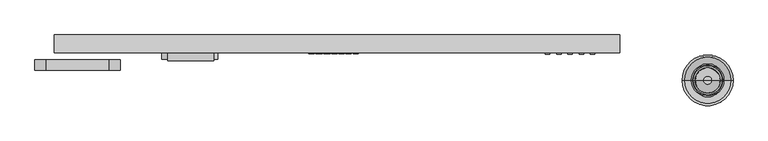
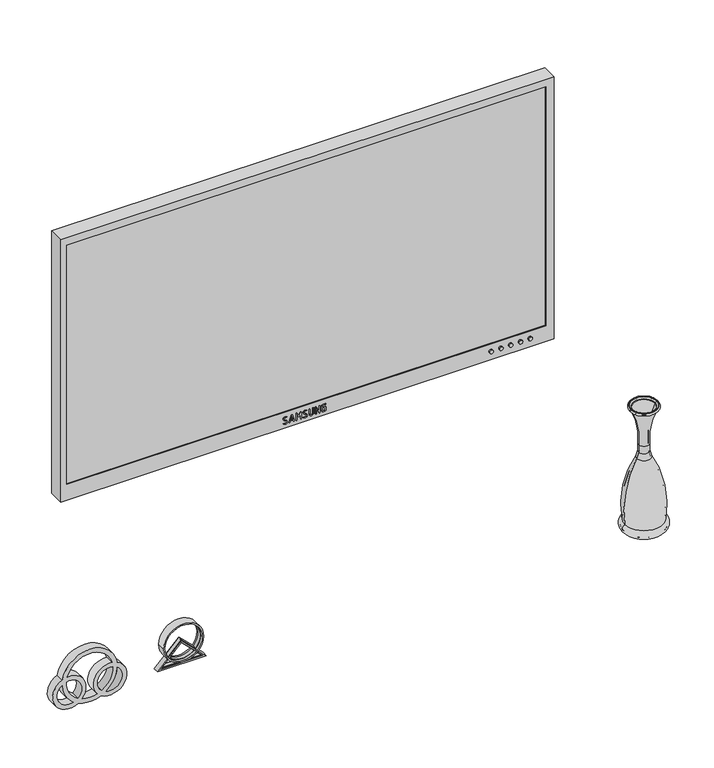
"""IFC4 building model written with IfcOpenShell, lengths in millimetres: furniture geometry."""

from ifc_helpers import new_model, si_unit, point, frame, frame_2d, origin, place, context, project, spatial, polyline, circle_curve, ellipse_curve, trimmed, segment, composite_curve, outline, extrude, faceted_brep, source, transform, mapped, element, save
from ifc_brep_helpers import plane_surface, cylinder_surface, revolved_surface, advanced_brep


def furniture_f593881e(model_context):
    return source(origin(), model_context, "Body", "SolidModel", [
        advanced_brep(
        [(1619.2140368, -127.8036565, 1022.4850219), (1533.669479, -127.8036565, 1022.4850219), (1532.6909812, -127.8036565, 1028.7350001), (1620.1925345, -127.8036565, 1028.7350001), (1617.5743227, -127.8036565, 1022.2360813), (1535.309193, -127.8036565, 1022.2360813), (1616.2567383, -127.8036565, 1021.2783955), (1536.6267775, -127.8036565, 1021.2783955), (1593.5125539, -127.8036565, 899.7037334), (1559.3709618, -127.8036565, 899.7037334), (1593.5125539, -127.8036565, 874.0721871), (1559.3709618, -127.8036565, 874.0721871), (1598.9034231, -127.8036565, 853.9701278), (1553.9800927, -127.8036565, 853.9701278), (1638.1633362, -127.8036565, 641.294886), (1514.7201795, -127.8036565, 641.294886), (1640.3690284, -127.8036565, 613.767552), (1512.5144873, -127.8036565, 613.767552), (1576.4417579, -127.8036565, 613.767552), (1634.3411967, -127.8036565, 617.0820621), (1518.5423191, -127.8036565, 617.0820621), (1576.4417579, -127.8036565, 617.0820621), (1632.4749509, -127.8036565, 637.0427782), (1520.4085649, -127.8036565, 637.0427782), (1594.3579463, -127.8036565, 851.8571485), (1558.5255695, -127.8036565, 851.8571485), (1588.5125539, -127.8036565, 873.6724497), (1564.3709618, -127.8036565, 873.6724497), (1588.5125539, -127.8036565, 899.4734315), (1564.3709618, -127.8036565, 899.4734315), (1611.5170749, -127.8036565, 1023.1126524), (1541.3664409, -127.8036565, 1023.1126524), (1612.9045122, -127.8036565, 1024.5000897), (1539.9790036, -127.8036565, 1024.5000897), (1616.8480298, -127.8036565, 1028.5337475), (1536.035486, -127.8036565, 1028.5337475)],
        [
            (0, 1, circle_curve(frame((1576.4417579, -127.8036565, 1022.4850219), z_axis=(0.0, 0.0, 1.0), x_axis=(-1.0, 0.0, 0.0)), 42.7722789)),
            (1, 2, circle_curve(frame((1533.4520615, -127.8036565, 1025.652569), z_axis=(0.0, 1.0, 0.0), x_axis=(1.0, 0.0, 0.0)), 3.175)),
            (2, 3, circle_curve(frame((1576.4417579, -127.8036565, 1028.7350001), z_axis=(0.0, 0.0, -1.0), x_axis=(-1.0, 0.0, 0.0)), 43.7507767)),
            (3, 0, circle_curve(frame((1619.4314542, -127.8036565, 1025.652569), z_axis=(0.0, 1.0, 0.0), x_axis=(-1.0, 0.0, 0.0)), 3.175)),
            (1, 0, circle_curve(frame((1576.4417579, -127.8036565, 1022.4850219), z_axis=(0.0, 0.0, 1.0), x_axis=(-1.0, 0.0, 0.0)), 42.7722789)),
            (3, 2, circle_curve(frame((1576.4417579, -127.8036565, 1028.7350001), z_axis=(0.0, 0.0, -1.0), x_axis=(-1.0, 0.0, 0.0)), 43.7507767)),
            (4, 5, circle_curve(frame((1576.4417579, -127.8036565, 1022.2360813), z_axis=(0.0, 0.0, 1.0), x_axis=(-1.0, 0.0, 0.0)), 41.1325648)),
            (5, 1, circle_curve(frame((1576.9707974, -127.8036565, 1302.1760704), z_axis=(0.0, 1.0, 0.0), x_axis=(1.0, 0.0, 0.0)), 283.0231206)),
            (0, 4, circle_curve(frame((1575.9127183, -127.8036565, 1302.1760704), z_axis=(0.0, 1.0, 0.0), x_axis=(-1.0, 0.0, 0.0)), 283.0231206)),
            (5, 4, circle_curve(frame((1576.4417579, -127.8036565, 1022.2360813), z_axis=(0.0, 0.0, 1.0), x_axis=(-1.0, 0.0, 0.0)), 41.1325648)),
            (6, 7, circle_curve(frame((1576.4417579, -127.8036565, 1021.2783955), z_axis=(0.0, 0.0, 1.0), x_axis=(-1.0, 0.0, 0.0)), 39.8149804)),
            (7, 5, circle_curve(frame((1535.0499641, -127.8036565, 1020.4942245), z_axis=(0.0, -1.0, 0.0), x_axis=(-1.0, 0.0, 0.0)), 1.7610408)),
            (4, 6, circle_curve(frame((1617.8335517, -127.8036565, 1020.4942245), z_axis=(0.0, -1.0, 0.0), x_axis=(1.0, 0.0, 0.0)), 1.7610408)),
            (7, 6, circle_curve(frame((1576.4417579, -127.8036565, 1021.2783955), z_axis=(0.0, 0.0, 1.0), x_axis=(-1.0, 0.0, 0.0)), 39.8149804)),
            (8, 9, circle_curve(frame((1576.4417579, -127.8036565, 899.7037334), z_axis=(0.0, 0.0, 1.0), x_axis=(-1.0, 0.0, 0.0)), 17.0707961)),
            (9, 7, circle_curve(frame((1334.1949035, -127.8036565, 920.6062281), z_axis=(0.0, -1.0, 0.0), x_axis=(1.0, 0.0, 0.0)), 226.1441389)),
            (6, 8, circle_curve(frame((1818.6886123, -127.8036565, 920.6062281), z_axis=(0.0, -1.0, 0.0), x_axis=(-1.0, 0.0, 0.0)), 226.1441389)),
            (9, 8, circle_curve(frame((1576.4417579, -127.8036565, 899.7037334), z_axis=(0.0, 0.0, 1.0), x_axis=(-1.0, 0.0, 0.0)), 17.0707961)),
            (10, 11, circle_curve(frame((1576.4417579, -127.8036565, 874.0721871), z_axis=(0.0, 0.0, 1.0), x_axis=(-1.0, 0.0, 0.0)), 17.0707961)),
            (11, 9),
            (8, 10),
            (11, 10, circle_curve(frame((1576.4417579, -127.8036565, 874.0721871), z_axis=(0.0, 0.0, 1.0), x_axis=(-1.0, 0.0, 0.0)), 17.0707961)),
            (12, 13, circle_curve(frame((1576.4417579, -127.8036565, 853.9701278), z_axis=(0.0, 0.0, 1.0), x_axis=(-1.0, 0.0, 0.0)), 22.4616652)),
            (13, 11, circle_curve(frame((1457.0512652, -127.8036565, 890.737891), z_axis=(0.0, -1.0, 0.0), x_axis=(1.0, 0.0, 0.0)), 103.6680569)),
            (10, 12, circle_curve(frame((1695.8322506, -127.8036565, 890.737891), z_axis=(0.0, -1.0, 0.0), x_axis=(-1.0, 0.0, 0.0)), 103.6680569)),
            (13, 12, circle_curve(frame((1576.4417579, -127.8036565, 853.9701278), z_axis=(0.0, 0.0, 1.0), x_axis=(-1.0, 0.0, 0.0)), 22.4616652)),
            (14, 15, circle_curve(frame((1576.4417579, -127.8036565, 641.294886), z_axis=(0.0, 0.0, 1.0), x_axis=(-1.0, 0.0, 0.0)), 61.7215784)),
            (15, 13, circle_curve(frame((1852.0874628, -127.8036565, 688.9781015), z_axis=(0.0, 1.0, 0.0), x_axis=(1.0, 0.0, 0.0)), 340.7203735)),
            (12, 14, circle_curve(frame((1300.7960529, -127.8036565, 688.9781015), z_axis=(0.0, 1.0, 0.0), x_axis=(-1.0, 0.0, 0.0)), 340.7203735)),
            (15, 14, circle_curve(frame((1576.4417579, -127.8036565, 641.294886), z_axis=(0.0, 0.0, 1.0), x_axis=(-1.0, 0.0, 0.0)), 61.7215784)),
            (16, 17, circle_curve(frame((1576.4417579, -127.8036565, 613.767552), z_axis=(0.0, 0.0, 1.0), x_axis=(-1.0, 0.0, 0.0)), 63.9272705)),
            (17, 15, circle_curve(frame((1519.5200125, -127.8036565, 627.058253), z_axis=(0.0, 1.0, 0.0), x_axis=(1.0, 0.0, 0.0)), 15.0239847)),
            (14, 16, circle_curve(frame((1633.3635033, -127.8036565, 627.058253), z_axis=(0.0, 1.0, 0.0), x_axis=(-1.0, 0.0, 0.0)), 15.0239847)),
            (17, 16, circle_curve(frame((1576.4417579, -127.8036565, 613.767552), z_axis=(0.0, 0.0, 1.0), x_axis=(-1.0, 0.0, 0.0)), 63.9272705)),
            (18, 17),
            (16, 18),
            (19, 20, circle_curve(frame((1576.4417579, -127.8036565, 617.0820621), z_axis=(0.0, 0.0, 1.0), x_axis=(-1.0, 0.0, 0.0)), 57.8994388)),
            (20, 21),
            (21, 19),
            (20, 19, circle_curve(frame((1576.4417579, -127.8036565, 617.0820621), z_axis=(0.0, 0.0, 1.0), x_axis=(-1.0, 0.0, 0.0)), 57.8994388)),
            (22, 23, circle_curve(frame((1576.4417579, -127.8036565, 637.0427782), z_axis=(0.0, 0.0, 1.0), x_axis=(-1.0, 0.0, 0.0)), 56.033193)),
            (23, 20, circle_curve(frame((1519.5200125, -127.8036565, 627.058253), z_axis=(0.0, -1.0, 0.0), x_axis=(1.0, 0.0, 0.0)), 10.0239847)),
            (19, 22, circle_curve(frame((1633.3635033, -127.8036565, 627.058253), z_axis=(0.0, -1.0, 0.0), x_axis=(-1.0, 0.0, 0.0)), 10.0239847)),
            (23, 22, circle_curve(frame((1576.4417579, -127.8036565, 637.0427782), z_axis=(0.0, 0.0, 1.0), x_axis=(-1.0, 0.0, 0.0)), 56.033193)),
            (24, 25, circle_curve(frame((1576.4417579, -127.8036565, 851.8571485), z_axis=(0.0, 0.0, 1.0), x_axis=(-1.0, 0.0, 0.0)), 17.9161884)),
            (25, 23, circle_curve(frame((1852.0874628, -127.8036565, 688.9781015), z_axis=(0.0, -1.0, 0.0), x_axis=(1.0, 0.0, 0.0)), 335.7203735)),
            (22, 24, circle_curve(frame((1300.7960529, -127.8036565, 688.9781015), z_axis=(0.0, -1.0, 0.0), x_axis=(-1.0, 0.0, 0.0)), 335.7203735)),
            (25, 24, circle_curve(frame((1576.4417579, -127.8036565, 851.8571485), z_axis=(0.0, 0.0, 1.0), x_axis=(-1.0, 0.0, 0.0)), 17.9161884)),
            (26, 27, circle_curve(frame((1576.4417579, -127.8036565, 873.6724497), z_axis=(0.0, 0.0, 1.0), x_axis=(-1.0, 0.0, 0.0)), 12.0707961)),
            (27, 25, circle_curve(frame((1457.0512652, -127.8036565, 890.737891), z_axis=(0.0, 1.0, 0.0), x_axis=(1.0, 0.0, 0.0)), 108.6680569)),
            (24, 26, circle_curve(frame((1695.8322506, -127.8036565, 890.737891), z_axis=(0.0, 1.0, 0.0), x_axis=(-1.0, 0.0, 0.0)), 108.6680569)),
            (27, 26, circle_curve(frame((1576.4417579, -127.8036565, 873.6724497), z_axis=(0.0, 0.0, 1.0), x_axis=(-1.0, 0.0, 0.0)), 12.0707961)),
            (28, 29, circle_curve(frame((1576.4417579, -127.8036565, 899.4734315), z_axis=(0.0, 0.0, 1.0), x_axis=(-1.0, 0.0, 0.0)), 12.0707961)),
            (29, 27),
            (26, 28),
            (29, 28, circle_curve(frame((1576.4417579, -127.8036565, 899.4734315), z_axis=(0.0, 0.0, 1.0), x_axis=(-1.0, 0.0, 0.0)), 12.0707961)),
            (30, 31, circle_curve(frame((1576.4417579, -127.8036565, 1023.1126524), z_axis=(0.0, 0.0, 1.0), x_axis=(-1.0, 0.0, 0.0)), 35.075317)),
            (31, 29, circle_curve(frame((1334.1949035, -127.8036565, 920.6062281), z_axis=(0.0, 1.0, 0.0), x_axis=(1.0, 0.0, 0.0)), 231.1441389)),
            (28, 30, circle_curve(frame((1818.6886123, -127.8036565, 920.6062281), z_axis=(0.0, 1.0, 0.0), x_axis=(-1.0, 0.0, 0.0)), 231.1441389)),
            (31, 30, circle_curve(frame((1576.4417579, -127.8036565, 1023.1126524), z_axis=(0.0, 0.0, 1.0), x_axis=(-1.0, 0.0, 0.0)), 35.075317)),
            (32, 33, circle_curve(frame((1576.4417579, -127.8036565, 1024.5000897), z_axis=(0.0, 0.0, 1.0), x_axis=(-1.0, 0.0, 0.0)), 36.4627543)),
            (33, 31),
            (30, 32),
            (33, 32, circle_curve(frame((1576.4417579, -127.8036565, 1024.5000897), z_axis=(0.0, 0.0, 1.0), x_axis=(-1.0, 0.0, 0.0)), 36.4627543)),
            (34, 35, circle_curve(frame((1576.4417579, -127.8036565, 1028.5337475), z_axis=(0.0, 0.0, 1.0), x_axis=(-1.0, 0.0, 0.0)), 40.4062719)),
            (35, 33, circle_curve(frame((1535.7876985, -127.8036565, 1024.3469724), z_axis=(0.0, 1.0, 0.0), x_axis=(-1.0, 0.0, 0.0)), 4.1941011)),
            (32, 34, circle_curve(frame((1617.0958173, -127.8036565, 1024.3469724), z_axis=(0.0, 1.0, 0.0), x_axis=(1.0, 0.0, 0.0)), 4.1941011)),
            (35, 34, circle_curve(frame((1576.4417579, -127.8036565, 1028.5337475), z_axis=(0.0, 0.0, 1.0), x_axis=(-1.0, 0.0, 0.0)), 40.4062719)),
            (2, 35, circle_curve(frame((1636.2916403, -127.8036565, 2722.5250067), z_axis=(0.0, -1.0, 0.0), x_axis=(1.0, 0.0, 0.0)), 1696.9554157)),
            (34, 3, circle_curve(frame((1516.5918754, -127.8036565, 2722.5250067), z_axis=(0.0, -1.0, 0.0), x_axis=(-1.0, 0.0, 0.0)), 1696.9554157)),
        ],
        [
            revolved_surface(trimmed(ellipse_curve(frame((1533.4520615, -127.8036565, 1025.652569), z_axis=(0.0, -1.0, 0.0), x_axis=(1.0, 0.0, 0.0)), 3.175, 3.175), [point((1532.6909812, -127.8036565, 1028.7350001))], [point((1533.669479, -127.8036565, 1022.4850219))], True, "CARTESIAN"), (1576.4417579, -127.8036565, 620.0444967), (0.0, 0.0, -1.0)),
            revolved_surface(trimmed(ellipse_curve(frame((1576.9707974, -127.8036565, 1302.1760704), z_axis=(0.0, -1.0, 0.0), x_axis=(1.0, 0.0, 0.0)), 283.0231206, 283.0231206), [point((1533.669479, -127.8036565, 1022.4850219))], [point((1535.309193, -127.8036565, 1022.2360813))], True, "CARTESIAN"), (1576.4417579, -127.8036565, 620.0444967), (0.0, 0.0, -1.0)),
            revolved_surface(trimmed(ellipse_curve(frame((1535.0499641, -127.8036565, 1020.4942245), z_axis=(0.0, 1.0, 0.0), x_axis=(-1.0, 0.0, 0.0)), 1.7610408, 1.7610408), [point((1535.309193, -127.8036565, 1022.2360813))], [point((1536.6267775, -127.8036565, 1021.2783955))], True, "CARTESIAN"), (1576.4417579, -127.8036565, 620.0444967), (0.0, 0.0, -1.0)),
            revolved_surface(trimmed(ellipse_curve(frame((1334.1949035, -127.8036565, 920.6062281), z_axis=(0.0, 1.0, 0.0), x_axis=(1.0, 0.0, 0.0)), 226.1441389, 226.1441389), [point((1536.6814689, -127.8036565, 1021.3055943))], [point((1559.3709618, -127.8036565, 899.7037334))], True, "CARTESIAN"), (1576.4417579, -127.8036565, 620.0444967), (0.0, 0.0, -1.0)),
            cylinder_surface(frame((1576.4417579, -127.8036565, 620.0444967), z_axis=(0.0, 0.0, -1.0), x_axis=(-1.0, 0.0, 0.0)), 17.0707961),
            revolved_surface(trimmed(ellipse_curve(frame((1457.0512652, -127.8036565, 890.737891), z_axis=(0.0, 1.0, 0.0), x_axis=(1.0, 0.0, 0.0)), 103.6680569, 103.6680569), [point((1559.3709618, -127.8036565, 874.0721871))], [point((1553.9800927, -127.8036565, 853.9701278))], True, "CARTESIAN"), (1576.4417579, -127.8036565, 620.0444967), (0.0, 0.0, -1.0)),
            revolved_surface(trimmed(ellipse_curve(frame((1852.0874628, -127.8036565, 688.9781015), z_axis=(0.0, -1.0, 0.0), x_axis=(1.0, 0.0, 0.0)), 340.7203735, 340.7203735), [point((1553.9800927, -127.8036565, 853.9701278))], [point((1514.7201795, -127.8036565, 641.294886))], True, "CARTESIAN"), (1576.4417579, -127.8036565, 620.0444967), (0.0, 0.0, -1.0)),
            revolved_surface(trimmed(ellipse_curve(frame((1519.5200125, -127.8036565, 627.058253), z_axis=(0.0, -1.0, 0.0), x_axis=(1.0, 0.0, 0.0)), 15.0239847, 15.0239847), [point((1514.7201795, -127.8036565, 641.294886))], [point((1512.5144873, -127.8036565, 613.767552))], True, "CARTESIAN"), (1576.4417579, -127.8036565, 620.0444967), (0.0, 0.0, -1.0)),
            plane_surface(frame((1576.4417579, -127.8036565, 613.767552), z_axis=(0.0, 0.0, -1.0), x_axis=(-1.0, 0.0, 0.0))),
            plane_surface(frame((1576.4417579, -127.8036565, 617.0820621), z_axis=(0.0, 0.0, 1.0), x_axis=(-1.0, 0.0, 0.0))),
            revolved_surface(trimmed(ellipse_curve(frame((1519.5200125, -127.8036565, 627.058253), z_axis=(0.0, 1.0, 0.0), x_axis=(1.0, 0.0, 0.0)), 10.0239847, 10.0239847), [point((1518.5423191, -127.8036565, 617.0820621))], [point((1520.4085649, -127.8036565, 637.0427782))], True, "CARTESIAN"), (1576.4417579, -127.8036565, 620.0444967), (0.0, 0.0, -1.0)),
            revolved_surface(trimmed(ellipse_curve(frame((1852.0874628, -127.8036565, 688.9781015), z_axis=(0.0, 1.0, 0.0), x_axis=(1.0, 0.0, 0.0)), 335.7203735, 335.7203735), [point((1520.4085649, -127.8036565, 637.0427782))], [point((1558.5255695, -127.8036565, 851.8571485))], True, "CARTESIAN"), (1576.4417579, -127.8036565, 620.0444967), (0.0, 0.0, -1.0)),
            revolved_surface(trimmed(ellipse_curve(frame((1457.0512652, -127.8036565, 890.737891), z_axis=(0.0, -1.0, 0.0), x_axis=(1.0, 0.0, 0.0)), 108.6680569, 108.6680569), [point((1558.5255695, -127.8036565, 851.8571485))], [point((1564.3709618, -127.8036565, 873.6724497))], True, "CARTESIAN"), (1576.4417579, -127.8036565, 620.0444967), (0.0, 0.0, -1.0)),
            revolved_surface(polyline([(1564.3709618, -127.8036565, 873.6724497), (1564.3709618, -127.8036565, 899.4734315)]), (1576.4417579, -127.8036565, 620.0444967), (0.0, 0.0, -1.0)),
            revolved_surface(trimmed(ellipse_curve(frame((1334.1949035, -127.8036565, 920.6062281), z_axis=(0.0, -1.0, 0.0), x_axis=(1.0, 0.0, 0.0)), 231.1441389, 231.1441389), [point((1564.3709618, -127.8036565, 899.4734315))], [point((1541.3664409, -127.8036565, 1023.1126524))], True, "CARTESIAN"), (1576.4417579, -127.8036565, 620.0444967), (0.0, 0.0, -1.0)),
            revolved_surface(polyline([(1541.3664409, -127.8036565, 1023.1126524), (1539.9790036, -127.8036565, 1024.5000897)]), (1576.4417579, -127.8036565, 620.0444967), (0.0, 0.0, -1.0)),
            revolved_surface(trimmed(ellipse_curve(frame((1535.7876985, -127.8036565, 1024.3469724), z_axis=(0.0, -1.0, 0.0), x_axis=(-1.0, 0.0, 0.0)), 4.1941011, 4.1941011), [point((1539.9790036, -127.8036565, 1024.5000897))], [point((1536.035486, -127.8036565, 1028.5337475))], True, "CARTESIAN"), (1576.4417579, -127.8036565, 620.0444967), (0.0, 0.0, -1.0)),
            revolved_surface(trimmed(ellipse_curve(frame((1636.2916403, -127.8036565, 2722.5250067), z_axis=(0.0, 1.0, 0.0), x_axis=(1.0, 0.0, 0.0)), 1696.9554157, 1696.9554157), [point((1536.035486, -127.8036565, 1028.5337475))], [point((1532.6909812, -127.8036565, 1028.7350001))], True, "CARTESIAN"), (1576.4417579, -127.8036565, 620.0444967), (0.0, 0.0, -1.0)),
        ],
        [
            (0, [[1, 2, 3, 4]]),
            (0, [[5, -4, 6, -2]]),
            (1, [[7, 8, -1, 9]]),
            (1, [[10, -9, -5, -8]]),
            (2, [[11, 12, -7, 13]]),
            (2, [[14, -13, -10, -12]]),
            (3, [[15, 16, -11, 17]]),
            (3, [[18, -17, -14, -16]]),
            (4, [[19, 20, -15, 21]]),
            (4, [[22, -21, -18, -20]]),
            (5, [[23, 24, -19, 25]]),
            (5, [[26, -25, -22, -24]]),
            (6, [[27, 28, -23, 29]]),
            (6, [[30, -29, -26, -28]]),
            (7, [[31, 32, -27, 33]]),
            (7, [[34, -33, -30, -32]]),
            (8, [[35, -31, 36]]),
            (8, [[-36, -34, -35]]),
            (9, [[37, 38, 39]]),
            (9, [[40, -39, -38]]),
            (10, [[41, 42, -37, 43]]),
            (10, [[44, -43, -40, -42]]),
            (11, [[45, 46, -41, 47]]),
            (11, [[48, -47, -44, -46]]),
            (12, [[49, 50, -45, 51]]),
            (12, [[52, -51, -48, -50]]),
            (13, [[53, 54, -49, 55]]),
            (13, [[56, -55, -52, -54]]),
            (14, [[57, 58, -53, 59]]),
            (14, [[60, -59, -56, -58]]),
            (15, [[61, 62, -57, 63]]),
            (15, [[64, -63, -60, -62]]),
            (16, [[65, 66, -61, 67]]),
            (16, [[68, -67, -64, -66]]),
            (17, [[-3, 69, -65, 70]]),
            (17, [[-6, -70, -68, -69]]),
        ],
    ),
        extrude(outline(composite_curve([segment(trimmed(circle_curve(frame_2d((1325.8720241, 1250.7088706)), 6.35), [point((1325.8720241, 1244.3588706))], [point((1325.8720241, 1257.0588706))], False, "CARTESIAN"), True, "CONTINUOUS"), segment(trimmed(circle_curve(frame_2d((1325.8720241, 1250.7088706)), 6.35), [point((1325.8720241, 1257.0588706))], [point((1325.8720241, 1244.3588706))], False, "CARTESIAN"), True, "CONTINUOUS")], self_intersect=False)), frame((0.0, -54.8067883, 0.0), z_axis=(0.0, 1.0, 0.0), x_axis=(0.0, 0.0, 1.0)), (0.0, 0.0, 1.0), 4.4067883),
        extrude(outline(composite_curve([segment(trimmed(circle_curve(frame_2d((1325.8720241, 1218.9588706)), 6.35), [point((1325.8720241, 1212.6088706))], [point((1325.8720241, 1225.3088706))], False, "CARTESIAN"), True, "CONTINUOUS"), segment(trimmed(circle_curve(frame_2d((1325.8720241, 1218.9588706)), 6.35), [point((1325.8720241, 1225.3088706))], [point((1325.8720241, 1212.6088706))], False, "CARTESIAN"), True, "CONTINUOUS")], self_intersect=False)), frame((0.0, -54.8067883, 0.0), z_axis=(0.0, 1.0, 0.0), x_axis=(0.0, 0.0, 1.0)), (0.0, 0.0, 1.0), 4.4067883),
        extrude(outline(composite_curve([segment(trimmed(circle_curve(frame_2d((1325.8720241, 1187.2088706)), 6.35), [point((1325.8720241, 1180.8588706))], [point((1325.8720241, 1193.5588706))], False, "CARTESIAN"), True, "CONTINUOUS"), segment(trimmed(circle_curve(frame_2d((1325.8720241, 1187.2088706)), 6.35), [point((1325.8720241, 1193.5588706))], [point((1325.8720241, 1180.8588706))], False, "CARTESIAN"), True, "CONTINUOUS")], self_intersect=False)), frame((0.0, -54.8067883, 0.0), z_axis=(0.0, 1.0, 0.0), x_axis=(0.0, 0.0, 1.0)), (0.0, 0.0, 1.0), 4.4067883),
        extrude(outline(composite_curve([segment(trimmed(circle_curve(frame_2d((1325.8720241, 1155.4588706)), 6.35), [point((1325.8720241, 1149.1088706))], [point((1325.8720241, 1161.8088706))], False, "CARTESIAN"), True, "CONTINUOUS"), segment(trimmed(circle_curve(frame_2d((1325.8720241, 1155.4588706)), 6.35), [point((1325.8720241, 1161.8088706))], [point((1325.8720241, 1149.1088706))], False, "CARTESIAN"), True, "CONTINUOUS")], self_intersect=False)), frame((0.0, -54.8067883, 0.0), z_axis=(0.0, 1.0, 0.0), x_axis=(0.0, 0.0, 1.0)), (0.0, 0.0, 1.0), 4.4067883),
        extrude(outline(composite_curve([segment(trimmed(circle_curve(frame_2d((1325.8720241, 1123.7088706)), 6.35), [point((1325.8720241, 1117.3588706))], [point((1325.8720241, 1130.0588706))], False, "CARTESIAN"), True, "CONTINUOUS"), segment(trimmed(circle_curve(frame_2d((1325.8720241, 1123.7088706)), 6.35), [point((1325.8720241, 1130.0588706))], [point((1325.8720241, 1117.3588706))], False, "CARTESIAN"), True, "CONTINUOUS")], self_intersect=False)), frame((0.0, -54.8067883, 0.0), z_axis=(0.0, 1.0, 0.0), x_axis=(0.0, 0.0, 1.0)), (0.0, 0.0, 1.0), 4.4067883),
        extrude(outline(polyline([(1316.1268551, 463.7978544), (1321.5823636, 460.3153333), (1325.1046093, 453.6416044), (1328.3686453, 451.9334477), (1330.6693604, 452.8371818), (1331.6194398, 455.0054816), (1333.2018021, 461.5534159), (1334.5855415, 454.8995494), (1332.7251072, 450.347775), (1328.4679568, 448.5436172), (1322.6549271, 451.9864138), (1319.1326814, 458.6535218), (1316.2261665, 460.4080239), (1313.5646199, 459.4248407), (1312.5516432, 457.2697824), (1313.0150966, 454.4228544), (1312.4390903, 449.2321765), (1309.5855415, 457.3690939), (1311.5088731, 461.9076267), (1316.1268551, 463.7978544)])), frame((0.0, -52.4, 0.0), z_axis=(0.0, 1.0, 0.0), x_axis=(0.0, 0.0, 1.0)), (0.0, 0.0, 1.0), 2.0),
        extrude(outline(polyline([(1311.4360447, 486.3680345), (1333.6387725, 478.9991256), (1334.5855415, 477.3902803), (1333.5990479, 475.7615727), (1311.2407322, 468.3728015), (1309.5855415, 470.0213714), (1310.6779674, 471.5904922), (1315.5177449, 473.2589244), (1315.5177449, 481.5150155), (1310.6779674, 483.1834477), (1309.5855415, 484.7591892), (1311.4360447, 486.3680345)]), holes=[polyline([(1328.8850648, 477.3836595), (1318.4838466, 480.5748672), (1318.4838466, 474.2056934), (1328.8850648, 477.3836595)])]), frame((0.0, -52.4, 0.0), z_axis=(0.0, 1.0, 0.0), x_axis=(0.0, 0.0, 1.0)), (0.0, 0.0, 1.0), 2.0),
        extrude(outline(polyline([(1334.5855415, 506.9122612), (1334.042639, 505.3894858), (1324.9523318, 499.7883205), (1333.7778085, 494.306329), (1334.5855415, 492.6908629), (1333.3540797, 490.9164985), (1311.2407322, 490.9164985), (1309.5855415, 492.6114138), (1311.2407322, 494.306329), (1328.8916856, 494.306329), (1321.5823636, 498.3449943), (1320.648836, 499.8148036), (1321.5757428, 501.2647506), (1328.8916856, 505.3232782), (1311.2407322, 505.3232782), (1309.5855415, 507.0181934), (1311.2407322, 508.7131087), (1333.3540797, 508.7131087), (1334.5855415, 506.9122612)])), frame((0.0, -52.4, 0.0), z_axis=(0.0, 1.0, 0.0), x_axis=(0.0, 0.0, 1.0)), (0.0, 0.0, 1.0), 2.0),
        extrude(outline(polyline([(1316.1268551, 528.6283629), (1321.5823636, 525.1458417), (1325.1046093, 518.4721129), (1328.3686453, 516.7639561), (1330.6693604, 517.6676902), (1331.6194398, 519.83599), (1333.2018021, 526.3839244), (1334.5855415, 519.7300578), (1332.7251072, 515.1782835), (1328.4679568, 513.3741256), (1322.6549271, 516.8169222), (1319.1326814, 523.4840303), (1316.2261665, 525.2385324), (1313.5646199, 524.2553491), (1312.5516432, 522.1002909), (1313.0150966, 519.2533629), (1312.4390903, 514.062685), (1309.5855415, 522.1996023), (1311.5088731, 526.7381352), (1316.1268551, 528.6283629)])), frame((0.0, -52.4, 0.0), z_axis=(0.0, 1.0, 0.0), x_axis=(0.0, 0.0, 1.0)), (0.0, 0.0, 1.0), 2.0),
        extrude(outline(polyline([(1333.3540797, 548.5436172), (1334.5855415, 546.8487019), (1333.3607004, 545.1537866), (1317.4510076, 545.1537866), (1313.91221, 543.8594275), (1312.5516432, 540.9164985), (1313.9088996, 537.9702591), (1317.4510076, 536.6792104), (1333.3607004, 536.6792104), (1334.5855415, 534.9842951), (1333.3540797, 533.2893799), (1317.3848, 533.2893799), (1311.8663943, 535.5205769), (1309.5855415, 540.9164985), (1311.8697047, 546.3091097), (1317.3848, 548.5436172), (1333.3540797, 548.5436172)])), frame((0.0, -52.4, 0.0), z_axis=(0.0, 1.0, 0.0), x_axis=(0.0, 0.0, 1.0)), (0.0, 0.0, 1.0), 2.0),
        extrude(outline(polyline([(1316.4115479, 565.0690409), (1333.7049801, 556.5944646), (1334.5855415, 554.9525155), (1333.3540797, 553.2046341), (1311.2407322, 553.2046341), (1309.5855415, 554.8995494), (1311.2407322, 556.5944646), (1328.2031263, 556.5944646), (1310.4263784, 565.1153862), (1309.5855415, 566.684507), (1311.2407322, 568.4588714), (1333.3540797, 568.4588714), (1334.5855415, 566.7639561), (1333.3540797, 565.0690409), (1316.4115479, 565.0690409)])), frame((0.0, -52.4, 0.0), z_axis=(0.0, 1.0, 0.0), x_axis=(0.0, 0.0, 1.0)), (0.0, 0.0, 1.0), 2.0),
        extrude(outline(polyline([(1312.5516432, 579.5817527), (1313.5513784, 577.4664191), (1316.2063042, 576.5097189), (1328.3885076, 576.5097189), (1330.6759811, 577.4233841), (1331.6194398, 579.6479604), (1331.6194398, 586.7652803), (1333.3143551, 588.3741256), (1334.5855415, 586.7520388), (1334.5855415, 579.5486489), (1332.7284176, 574.9339773), (1328.4414737, 573.1198883), (1316.1533381, 573.1198883), (1311.5055627, 574.9968746), (1309.5855415, 579.5486489), (1309.5855415, 586.7520388), (1311.247353, 588.3741256), (1323.6016962, 588.3741256), (1324.8397788, 586.6792104), (1324.8397788, 582.951721), (1323.5685924, 581.3031511), (1321.8736771, 582.951721), (1321.8736771, 584.9842951), (1312.5516432, 584.9842951), (1312.5516432, 579.5817527)])), frame((0.0, -52.4, 0.0), z_axis=(0.0, 1.0, 0.0), x_axis=(0.0, 0.0, 1.0)), (0.0, 0.0, 1.0), 2.0),
        faceted_brep([(1328.1814975, 0.4, 2195.8179594), (1328.1814975, 0.4, 1295.8179594), (-271.8185025, 0.4, 1295.8179594), (-271.8185025, 0.4, 2195.8179594), (1328.1814975, -50.4, 2195.8179594), (-271.8185025, -50.4, 2195.8179594), (-271.8185025, -50.4, 1295.8179594), (1328.1814975, -50.4, 1295.8179594), (-252.2185025, -50.4, 2170.4179594), (1302.7814975, -50.4, 2170.4179594), (1302.7814975, -50.4, 1350.4179594), (-252.2185025, -50.4, 1350.4179594), (-252.2185025, -25.0, 2170.4179594), (-252.2185025, -25.0, 1350.4179594), (1302.7814975, -25.0, 1350.4179594), (1302.7814975, -25.0, 2170.4179594)], [[[0, 1, 2, 3]], [[4, 5, 6, 7], [8, 9, 10, 11]], [[1, 0, 4, 7]], [[2, 1, 7, 6]], [[3, 2, 6, 5]], [[0, 3, 5, 4]], [[12, 13, 14, 15]], [[12, 15, 9, 8]], [[15, 14, 10, 9]], [[14, 13, 11, 10]], [[13, 12, 8, 11]]]),
        extrude(outline(polyline([(-252.2185025, -25.0), (1302.7814975, -25.0), (1302.7814975, -47.4310152), (-252.2185025, -47.4310152), (-252.2185025, -25.0)])), frame((0.0, 0.0, 1350.4179594), z_axis=(0.0, 0.0, 1.0), x_axis=(1.0, 0.0, 0.0)), (0.0, 0.0, 1.0), 820.0),
        extrude(outline(composite_curve([segment(trimmed(circle_curve(frame_2d((708.3591962, -206.3567667)), 90.0), [point((626.3492387, -243.429221))], [point((626.3492387, -169.2843123))], False, "CARTESIAN"), True, "CONTINUOUS"), segment(trimmed(circle_curve(frame_2d((673.3591962, -140.7349884)), 55.0), [point((626.3492387, -169.2843123))], [point((723.2559723, -117.5981836))], False, "CARTESIAN"), True, "CONTINUOUS"), segment(trimmed(circle_curve(frame_2d((708.3591962, -206.3567667)), 90.0), [point((723.2559723, -117.5981836))], [point((723.2559723, -295.1153497))], False, "CARTESIAN"), True, "CONTINUOUS"), segment(trimmed(circle_curve(frame_2d((673.3591962, -271.9785449)), 55.0), [point((723.2559723, -295.1153497))], [point((626.3492387, -243.429221))], False, "CARTESIAN"), True, "CONTINUOUS")], self_intersect=False), holes=[composite_curve([segment(trimmed(circle_curve(frame_2d((673.3591962, -271.9785449)), 40.0), [point((635.4713772, -259.1522763))], [point((705.1168322, -296.2983426))], True, "CARTESIAN"), True, "CONTINUOUS"), segment(trimmed(circle_curve(frame_2d((708.3591962, -206.3567667)), 90.0), [point((705.1168322, -296.2983426))], [point((635.4713772, -259.1522763))], False, "CARTESIAN"), True, "CONTINUOUS")], self_intersect=False), composite_curve([segment(trimmed(circle_curve(frame_2d((708.3591962, -206.3567667)), 75.0), [point((643.9805972, -244.8326811))], [point((712.2687203, -281.2548015))], True, "CARTESIAN"), True, "CONTINUOUS"), segment(trimmed(circle_curve(frame_2d((673.3591962, -271.9785449)), 40.0), [point((712.2687203, -281.2548015))], [point((643.9805972, -244.8326811))], True, "CARTESIAN"), True, "CONTINUOUS")], self_intersect=False), composite_curve([segment(trimmed(circle_curve(frame_2d((673.3591962, -140.7349884)), 55.0), [point((727.940069, -133.9579447))], [point((637.3262501, -182.2876875))], False, "CARTESIAN"), True, "CONTINUOUS"), segment(trimmed(circle_curve(frame_2d((708.3591962, -206.3567667)), 75.0), [point((637.3262501, -182.2876875))], [point((637.3262501, -230.4258459))], True, "CARTESIAN"), True, "CONTINUOUS"), segment(trimmed(circle_curve(frame_2d((673.3591962, -271.9785449)), 55.0), [point((637.3262501, -230.4258459))], [point((727.940069, -278.7555886))], False, "CARTESIAN"), True, "CONTINUOUS"), segment(trimmed(circle_curve(frame_2d((708.3591962, -206.3567667)), 75.0), [point((727.940069, -278.7555886))], [point((727.940069, -133.9579447))], True, "CARTESIAN"), True, "CONTINUOUS")], self_intersect=False), composite_curve([segment(trimmed(circle_curve(frame_2d((708.3591962, -206.3567667)), 75.0), [point((712.2687203, -131.4587318))], [point((643.9805972, -167.8808522))], True, "CARTESIAN"), True, "CONTINUOUS"), segment(trimmed(circle_curve(frame_2d((673.3591962, -140.7349884)), 40.0), [point((643.9805972, -167.8808522))], [point((712.2687203, -131.4587318))], True, "CARTESIAN"), True, "CONTINUOUS")], self_intersect=False), composite_curve([segment(trimmed(circle_curve(frame_2d((673.3591962, -140.7349884)), 40.0), [point((705.1168322, -116.4151908))], [point((635.4713772, -153.5612571))], True, "CARTESIAN"), True, "CONTINUOUS"), segment(trimmed(circle_curve(frame_2d((708.3591962, -206.3567667)), 90.0), [point((635.4713772, -153.5612571))], [point((705.1168322, -116.4151908))], False, "CARTESIAN"), True, "CONTINUOUS")], self_intersect=False)]), frame((0.0, -99.1314487, 0.0), z_axis=(0.0, 1.0, 0.0), x_axis=(0.0, 0.0, 1.0)), (0.0, 0.0, 1.0), 28.8519128),
        extrude(outline(polyline([(623.5602389, 43.8328824), (623.5602389, 178.1831708), (690.7353831, 111.0080266), (623.5602389, 43.8328824)]), holes=[composite_curve([segment(trimmed(circle_curve(frame_2d((692.8097661, 114.1885233)), 60.0), [point((649.5309431, 72.6320138))], [point((646.5346539, 152.3803286))], False, "CARTESIAN"), True, "CONTINUOUS"), segment(polyline([(646.5346539, 152.3803286), (625.5602389, 173.3547437), (625.5602389, 48.6613095), (649.5309431, 72.6320138)]), True, "CONTINUOUS")], self_intersect=False), composite_curve([segment(polyline([(650.9454582, 74.0465288), (687.9069559, 111.0080266), (647.9555529, 150.9594296)]), True, "CONTINUOUS"), segment(trimmed(circle_curve(frame_2d((692.8097661, 114.1885233)), 58.0), [point((647.9555529, 150.9594296))], [point((650.9454582, 74.0465288))], True, "CARTESIAN"), True, "CONTINUOUS")], self_intersect=False)]), frame((0.0, -64.2744539, 0.0), z_axis=(0.0, 1.0, 0.0), x_axis=(0.0, 0.0, 1.0)), (0.0, 0.0, 1.0), 11.6685342),
        extrude(outline(composite_curve([segment(trimmed(circle_curve(frame_2d((692.8097661, 114.1885233)), 60.0), [point((651.3011728, 157.5133047))], [point((654.6694162, 67.8709919))], False, "CARTESIAN"), True, "CONTINUOUS"), segment(polyline([(654.6694162, 67.8709919), (697.8064509, 111.0080266), (651.3011728, 157.5133047)]), True, "CONTINUOUS")], self_intersect=False), holes=[composite_curve([segment(polyline([(654.1856833, 157.4572213), (700.634878, 111.0080266), (657.6712227, 68.0443712)]), True, "CONTINUOUS"), segment(trimmed(circle_curve(frame_2d((692.8097661, 114.1885233)), 58.0), [point((657.6712227, 68.0443712))], [point((654.1856833, 157.4572213))], True, "CARTESIAN"), True, "CONTINUOUS")], self_intersect=False)]), frame((0.0, -64.2744539, 0.0), z_axis=(0.0, 1.0, 0.0), x_axis=(0.0, 0.0, 1.0)), (0.0, 0.0, 1.0), 11.6685342),
        extrude(outline(polyline([(618.5602389, 31.7618146), (618.5602389, 190.2542386), (697.8064509, 111.0080266), (618.5602389, 31.7618146)]), holes=[polyline([(623.5602389, 43.8328824), (690.7353831, 111.0080266), (623.5602389, 178.1831708), (623.5602389, 43.8328824)])]), frame((0.0, -67.8308187, 0.0), z_axis=(0.0, 1.0, 0.0), x_axis=(0.0, 0.0, 1.0)), (0.0, 0.0, 1.0), 18.5563648),
        extrude(outline(composite_curve([segment(trimmed(circle_curve(frame_2d((692.8097661, 114.1885233)), 65.0), [point((692.8097661, 179.1885233))], [point((692.8097661, 49.1885233))], False, "CARTESIAN"), True, "CONTINUOUS"), segment(trimmed(circle_curve(frame_2d((692.8097661, 114.1885233)), 65.0), [point((692.8097661, 49.1885233))], [point((692.8097661, 179.1885233))], False, "CARTESIAN"), True, "CONTINUOUS")], self_intersect=False), holes=[composite_curve([segment(trimmed(circle_curve(frame_2d((692.8097661, 114.1885233)), 60.0), [point((692.8097661, 174.1885233))], [point((692.8097661, 54.1885233))], True, "CARTESIAN"), True, "CONTINUOUS"), segment(trimmed(circle_curve(frame_2d((692.8097661, 114.1885233)), 60.0), [point((692.8097661, 54.1885233))], [point((692.8097661, 174.1885233))], True, "CARTESIAN"), True, "CONTINUOUS")], self_intersect=False)]), frame((0.0, -72.8308187, 0.0), z_axis=(0.0, 1.0, 0.0), x_axis=(0.0, 0.0, 1.0)), (0.0, 0.0, 1.0), 28.8519128),
    ])


if __name__ == "__main__":
    model = new_model("IFC4")
    model_context = context("Model", 3, world=origin())
    ifc_project = project(units=[si_unit("LENGTHUNIT", "METRE", prefix="MILLI")], contexts=[model_context])
    site = spatial("IfcSite", under=ifc_project)
    building = spatial("IfcBuilding", under=site)
    placement = place(None, origin())
    furniture_shape = furniture_f593881e(model_context)
    element("IfcFurniture", 1, at=placement, inside=building, context=model_context, shape_type="MappedRepresentation", body=[
        mapped(furniture_shape, transform((0.0, 0.0, 0.0), x_axis=(1.0, 0.0, 0.0), y_axis=(0.0, 1.0, 0.0), z_axis=(0.0, 0.0, 1.0))),
    ])
    save(model, "model.ifc")

# Revit data of these elements
# Type
#   Default Elevation = 0
# Element 1 (IfcFurniture)
#   Materials on its faces: "Phase - Demo", "wood 2(1)", "Porcelain, Ivory", "silver", "lit", "Default(1)", "Default Wall", "light", "wood 2", "tv button", "Modern Cabinet", "tv body", "Default", "Poche(1)", "Base Material", "Glass", "gold", "Sculpture"
# Materials
#   "Phase - Demo": class "System", colour RGB 255 255 255, transparency 0, Cost = 0
#   "wood 2(1)": class "Generic", colour RGB 129 75 29, transparency 0, Cost = 0
#   "Porcelain, Ivory": class "Ceramic", colour RGB 120 120 120, transparency 0, Description = "Porcelain, ivory", Cost = 0
#   "silver": class "Generic", colour RGB 120 120 120, transparency 0, Cost = 0
#   "lit": class "Generic", colour RGB 120 120 120, transparency 0, Cost = 0
#   "Default(1)": colour RGB 255 255 255, transparency 0, Cost = 0
#   "Default Wall": colour RGB 255 255 255, transparency 0, Cost = 0
#   "light": colour RGB 127 127 127, transparency 0, Cost = 0
#   "wood 2": class "Generic", colour RGB 120 120 120, transparency 0, Cost = 0
#   "tv button": class "Generic", colour RGB 120 120 120, transparency 0, Cost = 0
#   "Modern Cabinet": colour RGB 143 95 62, transparency 0, Cost = 0
#   "tv body": class "System", colour RGB 0 0 255, transparency 0, Cost = 0
#   "Default": colour RGB 255 255 255, transparency 0
#   "Poche(1)": class "System", colour RGB 244 244 244, transparency 0, Cost = 0
#   "Base Material": class "Glass", colour RGB 172 172 172, transparency 0, Cost = 0
#   "Glass": class "Glass", colour RGB 218 227 224, transparency 0.85, Description = "Soda Lime Glass", Cost = 0
#   "gold": class "Generic", colour RGB 120 120 120, transparency 0, Cost = 0
#   "Sculpture": colour RGB 219 183 111, transparency 0, Cost = 0
